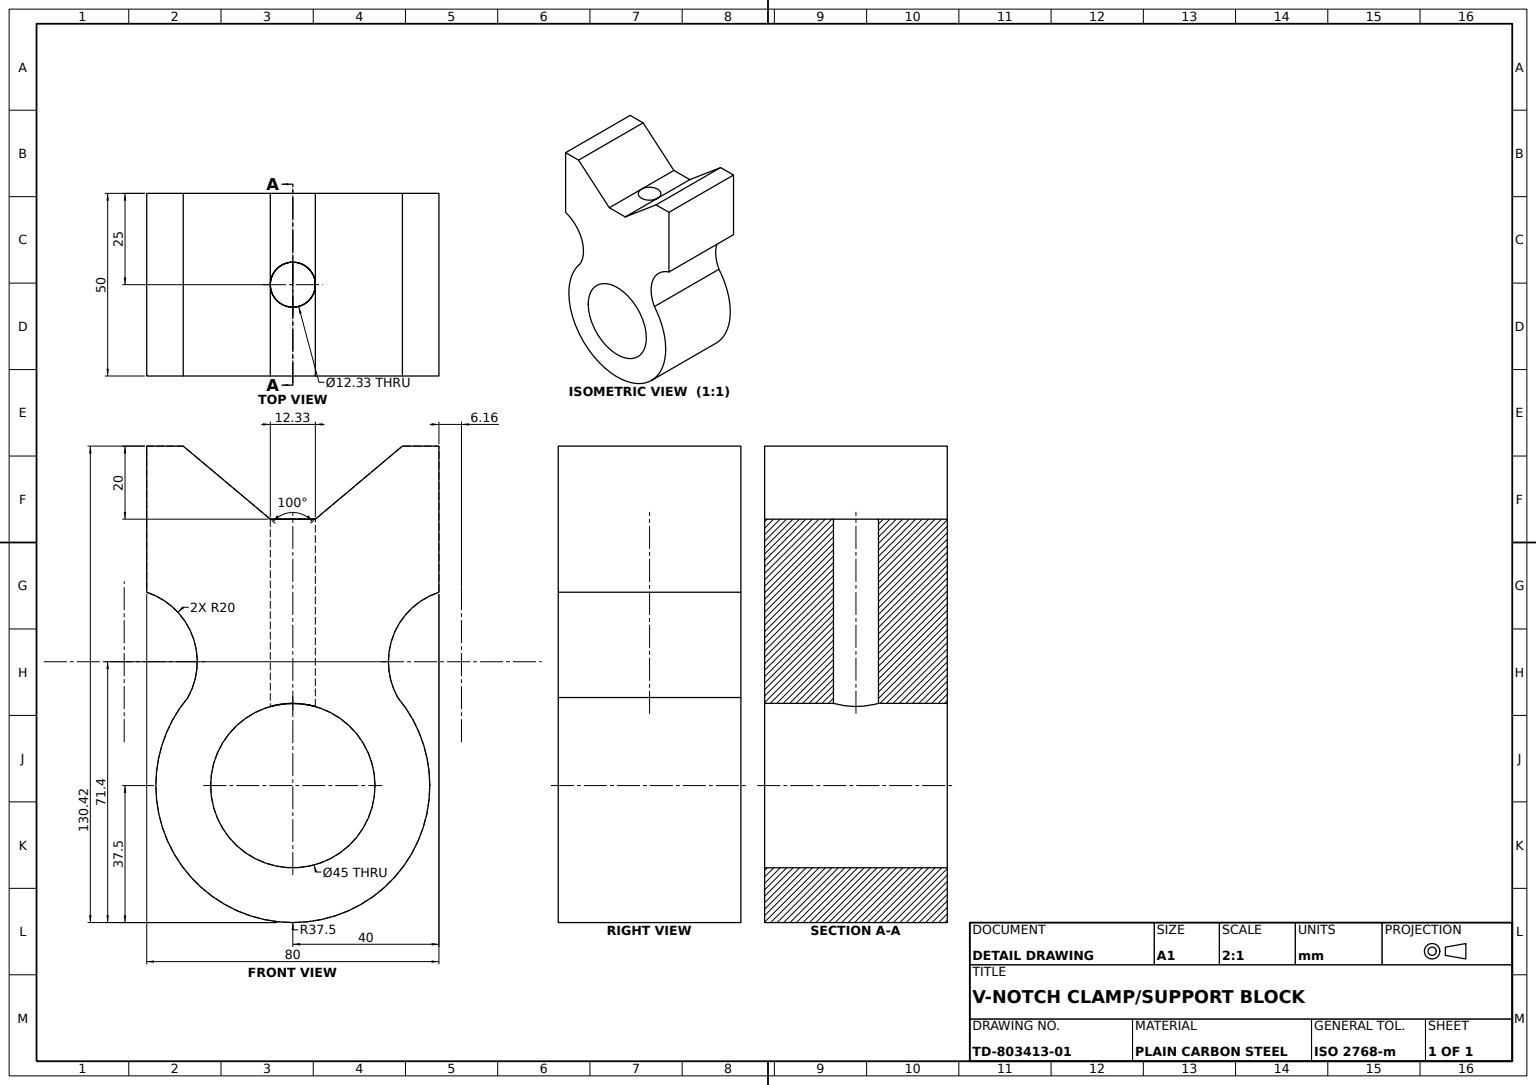
SolidWorks part; units mm, degrees
material "Plain Carbon Steel"
ref_plane "Front Plane" through (0, 0, 0) normal (0, 0, 1) x (1, 0, 0)
ref_plane "Top Plane" through (0, 0, 0) normal (0, 1, 0) x (1, 0, 0)
ref_plane "Right Plane" through (0, 0, 0) normal (1, 0, 0) x (0, 0, -1)
sketch "V-Block Profile Sketch" plane through (0, 0, 0) normal (0, 0, 1) x (1, 0, 0)
  line L0 (0, 0) -> (0, 94.4482) construction
  line L1 (0, 0) -> (-44.4364, 37.2866) construction
  line L2 (0, 0) -> (48.0131, 40.2878) construction
  line L7 (-40.0001, 52.9245) -> (-40.0001, 92.9245)
  line L8 (-40.0001, 92.9245) -> (-30.0001, 92.9245)
  line L12 (29.9999, 92.9245) -> (39.9999, 92.9245)
  line L13 (39.9999, 92.9245) -> (39.9999, 52.9245)
  line L14 (-30.0001, 92.9245) -> (-6.165, 72.9245)
  line L15 (-6.165, 72.9245) -> (6.1649, 72.9245)
  line L16 (6.1649, 72.9245) -> (29.9999, 92.9245)
  circle A0 centre (0, 0) radius 22.5
  arc A1 (-28.7267, 24.1045) -> (28.7267, 24.1045) centre (0, 0) ccw
  arc A2 (-28.7267, 24.1045) -> (-40.0001, 52.9245) centre (-46.1646, 33.8983) ccw
  arc A3 (28.7267, 24.1045) -> (39.9999, 52.9245) centre (46.1646, 33.8983) cw
  dimension "D1" = 45
  dimension "D2" = 75
  dimension "D5" = 20
  dimension "D6" = 20
  dimension "D3" = 50
  dimension "D4" = 50
  dimension "D7" = 40
  dimension "D8" = 40
  dimension "D9" = 70
  dimension "D10" = 50
  dimension "D11" = 12.3299
  dimension "D12" = 10
  dimension "D13" = 20
  dimension "D14" = 100
  dimension "D15" = 20
  dimension "D16" = 6.165
  dimension "D17" = 92.9245
extrude "V-Block Body" add sketch "V-Block Profile Sketch" along normal mid plane 50
sketch "Cross Hole Sketch" plane through (0, 72.9245, 0) normal (0, 1, 0) x (1, 0, 0)
  circle A0 centre (0, 0) radius 6.1649
  dimension "D1" = 12.3297
extrude "Cross Hole" cut sketch "Cross Hole Sketch" against normal blind 60
